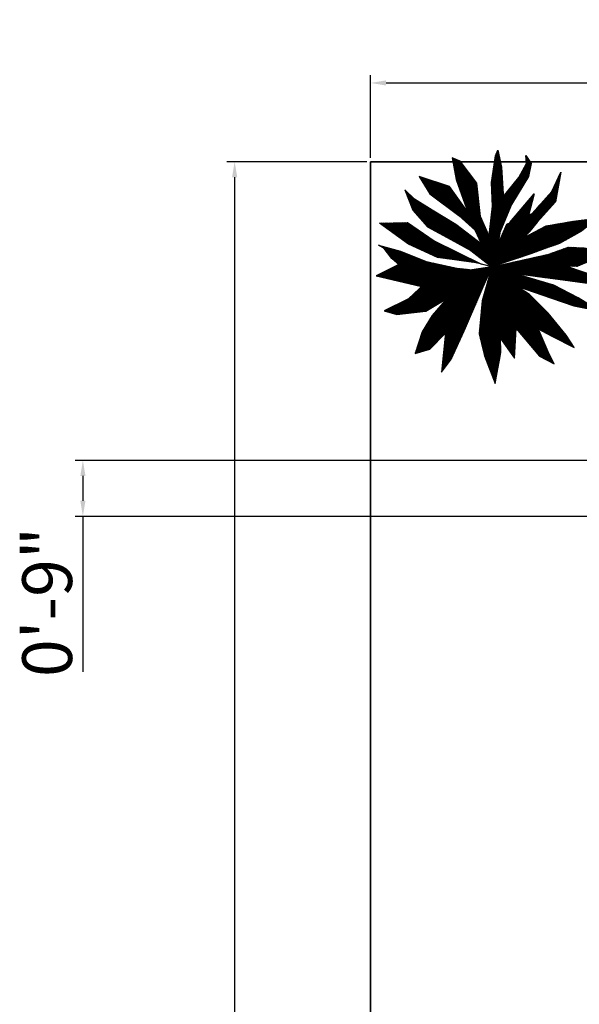
# Model space of a CAD drawing. Units: inches. Extents: x 1986 to 21484, y -1816 to 2016.
# Tile 8 of 85: x 1986 to 2076, y 1765 to 1924. Entities that reach past the tile are written whole.
import ezdxf

# ---------------------------------------------------------------- set-up
doc = ezdxf.new("R2010")
doc.units = ezdxf.units.IN
for name, color, linetype, lineweight in [('A-ANNO-DIMS', 2, 'Continuous', 18), ('C-PROP', 7, 'Continuous', 35), ('L-PLNT', 84, 'Continuous', 13), ('vfolhas', 114, 'Continuous', 5)]:
    doc.layers.add(name, color=color, linetype=linetype, lineweight=lineweight)
for name, color, linetype in [('vfolha', 72, 'Continuous'), ('vfolha2', 110, 'Continuous'), ('vfolhas2', 102, 'Continuous')]:
    doc.layers.add(name, color=color, linetype=linetype)
doc.styles.get("Standard").update_dxf_attribs({"font": 'arial.ttf'})
doc.dimstyles.new('ISO-25', dxfattribs={"dimtxt": 8, "dimasz": 2.5, "dimexe": 1.25, "dimexo": 0.625, "dimtad": 1, "dimdec": 1, "dimlunit": 3, "dimtxsty": 'Standard', "dimcen": 2.5, "dimadec": 0, "dimazin": 0, "dimtfac": 1, "dimtdec": 1, "dimtmove": 0, "dimatfit": 3, "dimfxl": 1, "dimarcsym": 0})
pattern_1 = [(45, (-2446.5133113, 50.986076), (-0.004419417382, 0.004419417382), [])]

# ---------------------------------------------------------------- blocks, each defined once
blk = doc.blocks.new('*D1')
at = {"layer": 'A-ANNO-DIMS', "color": 0, "lineweight": -2, "transparency": 16777216}
for p, q in [((2042.31, 1901.38), (2042.31, 1914.65)), ((2402.31, 1901.38), (2402.31, 1914.65)), ((2044.81, 1913.4), (2399.81, 1913.4))]:
    blk.add_line(p, q, dxfattribs=at)
at = {"layer": 'A-ANNO-DIMS', "color": 0, "transparency": 16777216}
for points in [[(2044.81, 1913.82), (2044.81, 1912.99), (2042.31, 1913.4)], [(2399.81, 1913.82), (2399.81, 1912.99), (2402.31, 1913.4)]]:
    blk.add_solid(points, dxfattribs=at)
at = {"layer": 'Defpoints', "color": 0, "transparency": 16777216}
for p in [(2402.31, 1913.4), (2042.31, 1900.75), (2402.31, 1900.75)]:
    blk.add_point(p, dxfattribs=at)
at = {"layer": 'A-ANNO-DIMS', "color": 0, "transparency": 16777216, "insert": (2222.31, 1918.12), "char_height": 8, "attachment_point": 5}
blk.add_mtext("30'", dxfattribs=at)
blk = doc.blocks.new('*D2')
at = {"layer": 'A-ANNO-DIMS', "color": 0, "lineweight": -2, "transparency": 16777216}
for p, q in [((2041.69, 1900.75), (2019.21, 1900.75)), ((2020.46, 1898.25), (2020.46, 1069.25)), ((2041.69, 1066.75), (2019.21, 1066.75))]:
    blk.add_line(p, q, dxfattribs=at)
at = {"layer": 'A-ANNO-DIMS', "color": 0, "transparency": 16777216}
for points in [[(2020.05, 1898.25), (2020.88, 1898.25), (2020.46, 1900.75)], [(2020.05, 1069.25), (2020.88, 1069.25), (2020.46, 1066.75)]]:
    blk.add_solid(points, dxfattribs=at)
at = {"layer": 'Defpoints', "color": 0, "transparency": 16777216}
for p in [(2042.31, 1900.75), (2020.46, 1066.75), (2042.31, 1066.75)]:
    blk.add_point(p, dxfattribs=at)
at = {"layer": 'A-ANNO-DIMS', "color": 0, "transparency": 16777216, "insert": (2015.75, 1483.75), "char_height": 8, "attachment_point": 5, "rotation": 90}
blk.add_mtext('69\'-6"', dxfattribs=at)
blk = doc.blocks.new('arbusto_PB_verde_grande')
at = {"layer": 'vfolha2'}
h = blk.add_hatch(dxfattribs=at)
h.set_pattern_fill('ANSI31', color=256, scale=0.05, style=0)
h.set_pattern_definition(pattern_1)
h.paths.add_polyline_path([(0.0294, 0.3565), (0.0003, 0.0905), (0.0263, -0.0393), (0.047, 0.0623), (0.0619, 0.0973), (0.0937, 0.2657), (0.0996, 0.4347), (0.0879, 0.6131), (0.0645, 0.7227), (0.0499, 0.6851), (0.0236, 0.5129)])
h.paths.add_polyline_path([(0.3011, 0.4379), (0.1423, 0.2487), (0.2669, 0.3002)])
h.paths.add_polyline_path([(0.38, 0.2282), (0.237, 0.1519), (0.1843, 0.0936), (0.1112, 0.0436), (0.0263, -0.0393), (0.2806, 0.0467), (0.3683, 0.078), (0.4676, 0.1124), (0.6107, 0.1938), (0.7159, 0.2782), (0.5581, 0.2595)])
h.paths.add_polyline_path([(0.561, -0.2944), (0.7275, -0.3257), (0.5902, -0.2412), (0.4296, -0.1598), (0.0263, -0.0393), (0.1492, -0.1411), (0.1884, -0.166), (0.415, -0.2444)])
h.paths.add_polyline_path([(-0.2743, -0.4478), (-0.3035, -0.7263), (-0.2392, -0.6417), (-0.1546, -0.4572), (0.0263, -0.0393), (-0.1633, -0.2538)])
h.paths.add_polyline_path([(-0.5196, -0.2474), (-0.6774, -0.3257), (-0.5956, -0.3507), (-0.4057, -0.3288), (-0.2101, -0.21), (0.0263, -0.0393), (-0.1487, -0.0659), (-0.3152, -0.091), (-0.4145, -0.1505)])
h.paths.add_polyline_path([(-0.5255, 0.2501), (-0.7095, 0.247), (-0.5196, 0.1093), (-0.3298, 0.0217), (-0.0757, -0.0128), (-0.0423, -0.0215), (-0.3502, 0.1312)])
h = blk.add_hatch(dxfattribs=at)
h.set_pattern_fill('ANSI31', color=256, scale=0.05, style=0)
h.set_pattern_definition(pattern_1)
h.paths.add_polyline_path([(-0.1896, 0.297), (-0.0855, 0.2019), (-0.1078, 0.2501), (-0.132, 0.3187), (-0.251, 0.4848), (-0.4495, 0.5505), (-0.3795, 0.4379)])
h.paths.add_polyline_path([(0.0791, -0.4071), (0.0821, -0.5063), (0.1726, -0.6355), (0.1843, -0.4415), (0.149, -0.2918), (0.0263, -0.0393), (0.0353, -0.2538)])
at = {"layer": 'vfolhas'}
h = blk.add_hatch(dxfattribs=at)
h.set_pattern_fill('ANSI31', color=256, scale=0.05, style=0)
h.set_pattern_definition(pattern_1)
h.paths.add_polyline_path([(-0.0728, 0.5067), (-0.1808, 0.6506), (-0.2334, 0.6725), (-0.2071, 0.5318), (-0.1078, 0.2501), (0.0263, -0.0393), (0.0003, 0.0905), (0.0082, 0.1624), (-0.0494, 0.2908)])
h.paths.add_polyline_path([(0.099, 0.4193), (0.0937, 0.2657), (0.0791, 0.1881), (0.1551, 0.369), (0.2661, 0.5505), (0.2836, 0.635), (0.2485, 0.6882), (0.2514, 0.635), (0.2018, 0.5443)])
h.paths.add_polyline_path([(0.1229, 0.2407), (0.047, 0.0623), (0.0263, -0.0393), (0.1112, 0.0436), (0.1843, 0.0936), (0.2748, 0.1938), (0.3215, 0.2532), (0.4413, 0.3847), (0.4763, 0.5787), (0.4179, 0.4535), (0.2894, 0.3095)])
h.paths.add_polyline_path([(0.5815, -0.0378), (0.7071, 0.0154), (0.7859, 0.0467), (0.748, 0.0655), (0.6282, 0.0842), (0.526, 0.0905), (0.3974, 0.0436), (0.0263, -0.0393), (0.2573, -0.0315), (0.4383, -0.0347)])
h.paths.add_polyline_path([(0.5202, -0.0365), (0.4383, -0.0347), (0.2573, -0.0315), (0.0263, -0.0393), (0.1796, -0.0852), (0.5377, -0.1317), (0.6954, -0.1536), (0.7859, -0.0785), (0.7041, -0.1004)])
h.paths.add_polyline_path([(0.2719, -0.2193), (0.1492, -0.1411), (0.0263, -0.0393), (0.1579, -0.3101), (0.2952, -0.4258), (0.4179, -0.4916), (0.564, -0.5667), (0.5114, -0.4853), (0.3946, -0.3414)])
h.paths.add_polyline_path([(-0.0582, -0.4759), (-0.0231, -0.6198), (0.047, -0.8013), (0.0849, -0.5979), (0.0791, -0.4071), (0.0353, -0.2538), (0.0263, -0.0393), (-0.0377, -0.26)])
h.paths.add_polyline_path([(-0.2422, 0.1405), (-0.1107, 0.0686), (0.0263, -0.0393), (-0.0423, 0.1087), (-0.2101, 0.2376), (-0.3649, 0.3314), (-0.4787, 0.4034), (-0.543, 0.4629), (-0.4904, 0.3314), (-0.3941, 0.2219)])
h = blk.add_hatch(dxfattribs=at)
h.set_pattern_fill('ANSI31', color=256, scale=0.05, style=0)
h.set_pattern_definition(pattern_1)
h.paths.add_polyline_path([(-0.5722, 0.0623), (-0.7153, 0.103), (-0.6774, 0.0811), (-0.6277, 0.0154), (-0.5635, -0.041), (-0.2646, -0.0834), (-0.1487, -0.0659), (-0.1015, -0.0588), (-0.2042, -0.0472), (-0.4028, -0.0034)])
h.paths.add_polyline_path([(-0.5635, -0.041), (-0.5828, -0.024), (-0.7299, -0.0973), (-0.4334, -0.1679), (-0.4145, -0.1505), (-0.3152, -0.091), (-0.2646, -0.0834)])
h.paths.add_polyline_path([(-0.2769, -0.4727), (-0.2743, -0.4478), (-0.1633, -0.2538), (0.0263, -0.0393), (-0.2101, -0.21), (-0.2672, -0.2447), (-0.3649, -0.357), (-0.4291, -0.4634), (-0.4759, -0.6043), (-0.3795, -0.576)])
h = blk.add_hatch(dxfattribs=at)
h.set_pattern_fill('ANSI31', color=256, scale=0.05, style=0)
h.set_pattern_definition(pattern_1)
h.paths.add_polyline_path([(0.3361, -0.623), (0.4325, -0.6731), (0.3946, -0.5948), (0.3303, -0.4446), (0.2952, -0.4258), (0.1579, -0.3101), (0.149, -0.2918), (0.1843, -0.4415)])
at = {"layer": 'vfolha'}
for p, q in [((0.0263, -0.0393), (-0.1487, -0.0659)), ((0.0263, -0.0393), (-0.0377, -0.26)), ((0.0353, -0.2538), (0.0263, -0.0393)), ((0.5202, -0.0365), (0.7041, -0.1004)), ((0.5377, -0.1317), (0.1796, -0.0852)), ((0.7859, -0.0785), (0.6954, -0.1536)), ((0.7041, -0.1004), (0.7859, -0.0785)), ((0.6954, -0.1536), (0.5377, -0.1317)), ((-0.2672, -0.2447), (-0.3649, -0.357)), ((0.0791, -0.4071), (0.0353, -0.2538)), ((0.3946, -0.3414), (0.2719, -0.2193)), ((-0.0377, -0.26), (-0.0582, -0.4759)), ((0.1579, -0.3101), (0.2952, -0.4258)), ((0.5114, -0.4853), (0.3946, -0.3414)), ((0.0849, -0.5979), (0.0791, -0.4071)), ((0.2952, -0.4258), (0.4179, -0.4916)), ((0.4179, -0.4916), (0.564, -0.5667)), ((0.564, -0.5667), (0.5114, -0.4853)), ((-0.0231, -0.6198), (0.047, -0.8013)), ((0.047, -0.8013), (0.0849, -0.5979))]:
    blk.add_line(p, q, dxfattribs=at)
at = {"layer": 'vfolha2'}
for p, q in [((0.0499, 0.6851), (0.0645, 0.7227)), ((0.0645, 0.7227), (0.0879, 0.6131)), ((0.0236, 0.5129), (0.0499, 0.6851)), ((0.0879, 0.6131), (0.0996, 0.4347)), ((-0.4495, 0.5505), (-0.3795, 0.4379)), ((-0.251, 0.4848), (-0.4495, 0.5505)), ((-0.132, 0.3187), (-0.251, 0.4848)), ((0.0294, 0.3565), (0.0236, 0.5129)), ((-0.3795, 0.4379), (-0.1896, 0.297)), ((0.0996, 0.4347), (0.0937, 0.2657)), ((0.1434, 0.2501), (0.3011, 0.4379)), ((0.3011, 0.4379), (0.2661, 0.297)), ((0.0003, 0.0905), (0.0294, 0.3565)), ((-0.1896, 0.297), (-0.0822, 0.1989)), ((0.38, 0.2282), (0.5581, 0.2595)), ((0.5581, 0.2595), (0.7159, 0.2782)), ((0.7159, 0.2782), (0.6107, 0.1938)), ((-0.7095, 0.247), (-0.5255, 0.2501)), ((-0.5196, 0.1093), (-0.7095, 0.247)), ((-0.5255, 0.2501), (-0.3502, 0.1312)), ((0.237, 0.1519), (0.38, 0.2282)), ((0.6107, 0.1938), (0.4676, 0.1124)), ((-0.3502, 0.1312), (-0.0423, -0.0215)), ((-0.3298, 0.0217), (-0.5196, 0.1093)), ((0.0263, -0.0393), (0.0003, 0.0905)), ((0.3683, 0.078), (0.2806, 0.0467)), ((-0.0757, -0.0128), (-0.3298, 0.0217)), ((0.2806, 0.0467), (0.0263, -0.0393)), ((-0.2101, -0.21), (0.0263, -0.0393)), ((0.0263, -0.0393), (-0.1633, -0.2538)), ((-0.1546, -0.4572), (0.0263, -0.0393)), ((0.4296, -0.1598), (0.0263, -0.0393)), ((0.0263, -0.0393), (0.1579, -0.3101)), ((-0.3152, -0.091), (-0.4145, -0.1505)), ((-0.1487, -0.0659), (-0.3152, -0.091)), ((-0.4145, -0.1505), (-0.5196, -0.2474)), ((0.1884, -0.166), (0.415, -0.2444)), ((0.5902, -0.2412), (0.4296, -0.1598)), ((-0.5196, -0.2474), (-0.6774, -0.3257)), ((-0.4057, -0.3288), (-0.2101, -0.21)), ((-0.1633, -0.2538), (-0.2743, -0.4478)), ((0.415, -0.2444), (0.561, -0.2944)), ((0.7275, -0.3257), (0.5902, -0.2412)), ((0.1843, -0.4415), (0.149, -0.2918)), ((0.561, -0.2944), (0.7275, -0.3257)), ((-0.6774, -0.3257), (-0.5956, -0.3507)), ((-0.5956, -0.3507), (-0.4057, -0.3288)), ((-0.2743, -0.4478), (-0.3035, -0.7263)), ((0.1726, -0.6355), (0.1843, -0.4415)), ((0.0821, -0.5063), (0.1726, -0.6355)), ((-0.3035, -0.7263), (-0.2392, -0.6417))]:
    blk.add_line(p, q, dxfattribs=at)
at = {"layer": 'vfolhas2'}
for p, q in [((-0.2334, 0.6725), (-0.2071, 0.5318)), ((-0.1808, 0.6506), (-0.2334, 0.6725)), ((-0.0728, 0.5067), (-0.1808, 0.6506)), ((0.2514, 0.635), (0.2485, 0.6882)), ((0.2485, 0.6882), (0.2836, 0.635)), ((0.2018, 0.5443), (0.2514, 0.635)), ((0.2836, 0.635), (0.2661, 0.5505)), ((-0.2071, 0.5318), (-0.1078, 0.2501)), ((0.099, 0.4193), (0.2018, 0.5443)), ((0.2661, 0.5505), (0.1551, 0.369)), ((0.4179, 0.4535), (0.4763, 0.5787)), ((0.4763, 0.5787), (0.4413, 0.3847)), ((-0.543, 0.4629), (-0.4904, 0.3314)), ((-0.4787, 0.4034), (-0.543, 0.4629)), ((-0.0494, 0.2908), (-0.0728, 0.5067)), ((0.2894, 0.3095), (0.4179, 0.4535)), ((-0.3649, 0.3314), (-0.4787, 0.4034)), ((-0.4904, 0.3314), (-0.3941, 0.2219)), ((-0.2101, 0.2376), (-0.3649, 0.3314)), ((0.1551, 0.369), (0.078, 0.1855)), ((0.4413, 0.3847), (0.3215, 0.2532)), ((0.0082, 0.1624), (-0.0494, 0.2908)), ((0.0937, 0.2657), (0.0619, 0.0973)), ((0.1229, 0.2407), (0.2894, 0.3095)), ((-0.3941, 0.2219), (-0.2422, 0.1405)), ((-0.0423, 0.1087), (-0.2101, 0.2376)), ((-0.1078, 0.2501), (0.0263, -0.0393)), ((0.047, 0.0623), (0.1229, 0.2407)), ((0.2748, 0.1938), (0.1843, 0.0936)), ((0.3215, 0.2532), (0.2748, 0.1938)), ((-0.2422, 0.1405), (-0.1107, 0.0686)), ((-0.6774, 0.0811), (-0.7153, 0.103)), ((-0.7153, 0.103), (-0.5722, 0.0623)), ((-0.6277, 0.0154), (-0.6774, 0.0811)), ((-0.1107, 0.0686), (0.0263, -0.0393)), ((0.1843, 0.0936), (0.1112, 0.0436)), ((0.4676, 0.1124), (0.3683, 0.078)), ((0.3974, 0.0436), (0.526, 0.0905)), ((0.526, 0.0905), (0.6282, 0.0842)), ((0.6282, 0.0842), (0.748, 0.0655)), ((0.748, 0.0655), (0.7859, 0.0467)), ((-0.5635, -0.041), (-0.6277, 0.0154)), ((-0.5722, 0.0623), (-0.4028, -0.0034)), ((0.0263, -0.0393), (0.047, 0.0623)), ((0.0263, -0.0393), (0.3974, 0.0436)), ((0.1112, 0.0436), (0.0263, -0.0393)), ((0.7071, 0.0154), (0.5815, -0.0378)), ((0.7859, 0.0467), (0.7071, 0.0154)), ((-0.5828, -0.024), (-0.7299, -0.0973)), ((-0.2646, -0.0834), (-0.5635, -0.041)), ((-0.4028, -0.0034), (-0.2042, -0.0472)), ((-0.2042, -0.0472), (-0.0983, -0.0591)), ((0.0263, -0.0393), (-0.0757, -0.0128)), ((0.2573, -0.0315), (0.0263, -0.0393)), ((0.1492, -0.1411), (0.0263, -0.0393)), ((0.4383, -0.0347), (0.2573, -0.0315)), ((0.5815, -0.0378), (0.4383, -0.0347)), ((-0.7299, -0.0973), (-0.4334, -0.1679)), ((0.2719, -0.2193), (0.1492, -0.1411)), ((-0.3649, -0.357), (-0.4291, -0.4634)), ((0.1843, -0.4415), (0.3361, -0.623)), ((0.3946, -0.5948), (0.329, -0.4417)), ((-0.4291, -0.4634), (-0.4759, -0.6043)), ((-0.3795, -0.576), (-0.2769, -0.4727)), ((-0.2392, -0.6417), (-0.1546, -0.4572)), ((-0.0582, -0.4759), (-0.0231, -0.6198)), ((-0.4759, -0.6043), (-0.3795, -0.576)), ((0.3361, -0.623), (0.4325, -0.6731)), ((0.4325, -0.6731), (0.3946, -0.5948))]:
    blk.add_line(p, q, dxfattribs=at)
blk = doc.blocks.new('*D135')
at = {"layer": 'A-ANNO-DIMS', "color": 0, "lineweight": -2, "transparency": 16777216}
for p, q in [((2077.69, 1852.75), (1994.81, 1852.75)), ((1996.06, 1850.25), (1996.06, 1846.25)), ((2086.69, 1843.75), (1994.81, 1843.75)), ((1996.06, 1843.75), (1996.06, 1818.74))]:
    blk.add_line(p, q, dxfattribs=at)
at = {"layer": 'A-ANNO-DIMS', "color": 0, "transparency": 16777216}
for points in [[(1995.65, 1850.25), (1996.48, 1850.25), (1996.06, 1852.75)], [(1995.65, 1846.25), (1996.48, 1846.25), (1996.06, 1843.75)]]:
    blk.add_solid(points, dxfattribs=at)
at = {"layer": 'Defpoints', "color": 0, "transparency": 16777216}
for p in [(2078.31, 1852.75), (1996.06, 1843.75), (2087.31, 1843.75)]:
    blk.add_point(p, dxfattribs=at)
at = {"layer": 'A-ANNO-DIMS', "color": 0, "transparency": 16777216, "insert": (1991.35, 1829.99), "char_height": 8, "attachment_point": 5, "rotation": 90}
blk.add_mtext('0\'-9"', dxfattribs=at)

msp = doc.modelspace()

# ---------------------------------------------------------------- linework, layer by layer
at = {"layer": 'C-PROP'}
msp.add_lwpolyline([(2042.31, 1900.75), (2402.31, 1900.75), (2402.31, 1066.75), (2042.31, 1066.75)], close=True, dxfattribs=at)

# ---------------------------------------------------------------- block references
at = {"layer": 'L-PLNT', "xscale": 24.60366729364114, "yscale": 24.60366729364114, "zscale": 24.60366729364114}
msp.add_blockref('arbusto_PB_verde_grande', (2061.18, 1884.81), dxfattribs=at)

# ---------------------------------------------------------------- dimensions: what is measured, and where the dimension line sits
at = {"layer": 'A-ANNO-DIMS'}
dim = msp.add_linear_dim(base=(2402.31, 1913.4), p1=(2042.31, 1900.75), p2=(2402.31, 1900.75), dimstyle='ISO-25', override={"dimclrd": 0, "dimclre": 0, "dimclrt": 0}, dxfattribs=at)
dim.commit()
dim.dimension.update_dxf_attribs({"geometry": '*D1', "text_midpoint": (2222.31, 1918.12)})
for base, p1, p2, override, picture, middle in [((2020.46, 1066.75), (2042.31, 1900.75), (2042.31, 1066.75), {"dimclrd": 0, "dimclre": 0, "dimclrt": 0}, '*D2', (2015.75, 1483.75)), ((1996.06, 1843.75), (2078.31, 1852.75), (2087.31, 1843.75), {"dimdec": 1, "dimlfac": 1, "dimrnd": 0, "dimzin": 1, "dimdsep": 46, "dimlunit": 4, "dimfrac": 2}, '*D135', (1991.35, 1829.99))]:
    dim = msp.add_linear_dim(base=base, p1=p1, p2=p2, angle=90, dimstyle='ISO-25', override=override, dxfattribs=at)
    dim.commit()
    dim.dimension.update_dxf_attribs({"geometry": picture, "text_midpoint": middle})

doc.saveas('drawing.dxf')
